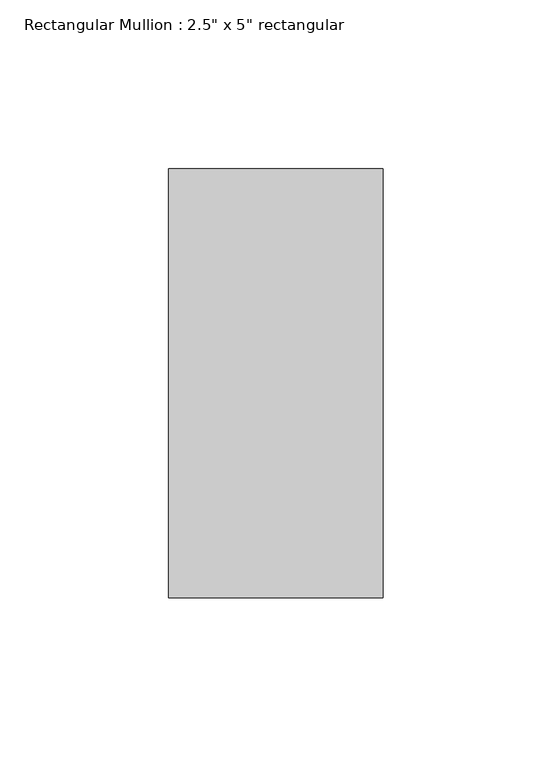
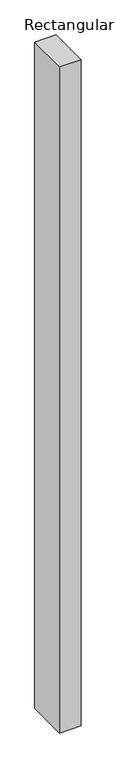
"""IFC4 building model written with IfcOpenShell, lengths in millimetres: member geometry."""

from ifc_helpers import new_model, si_unit, frame, origin, place, context, project, spatial, polyline, outline, extrude, source, transform, mapped, element, save


def member_1cdc6c9a(model_context):
    return source(origin(), model_context, "Body", "SweptSolid", [
        extrude(outline(polyline([(0.0, 63.5), (0.0, -63.5), (-63.5, -63.5), (-63.5, 63.5), (0.0, 63.5)])), frame((0.0, 0.0, -2080.6846597), z_axis=(0.0, 0.0, 1.0), x_axis=(1.0, 0.0, 0.0)), (0.0, 0.0, 1.0), 2080.6846597),
    ])


if __name__ == "__main__":
    model = new_model("IFC4")
    model_context = context("Model", 3, world=origin())
    ifc_project = project(units=[si_unit("LENGTHUNIT", "METRE", prefix="MILLI")], contexts=[model_context])
    site = spatial("IfcSite", under=ifc_project)
    building = spatial("IfcBuilding", under=site)
    placement = place(None, origin())
    member_shape = member_1cdc6c9a(model_context)
    element("IfcMember", 1, ObjectType="Rectangular Mullion : 2.5\" x 5\" rectangular", at=placement, inside=building, context=model_context, shape_type="MappedRepresentation", body=[
        mapped(member_shape, transform((0.0, 0.0, 0.0), x_axis=(1.0, 0.0, 0.0), y_axis=(0.0, 1.0, 0.0), z_axis=(0.0, 0.0, 1.0))),
    ])
    save(model, "model.ifc")

# Revit data of these elements
# Type "Rectangular Mullion : 2.5\" x 5\" rectangular"
#   built-in parameter 1007304 = 0.416667 (stored number, unit not read)
#   built-in parameter 1007301 = 0.104167 (stored number, unit not read)
#   built-in parameter 1007300 = 0.104167 (stored number, unit not read)
# Element 1 (IfcMember, "Rectangular Mullion : 2.5\" x 5\" rectangular")
#   Materials on its faces: "Aluminum"
# Materials
#   "Aluminum": class "Metal", colour RGB 247 247 247, transparency 0, Description = "Aluminum 6061", Cost = 0
